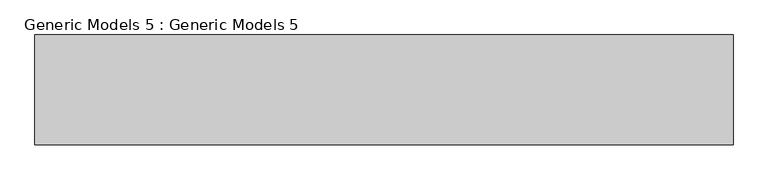
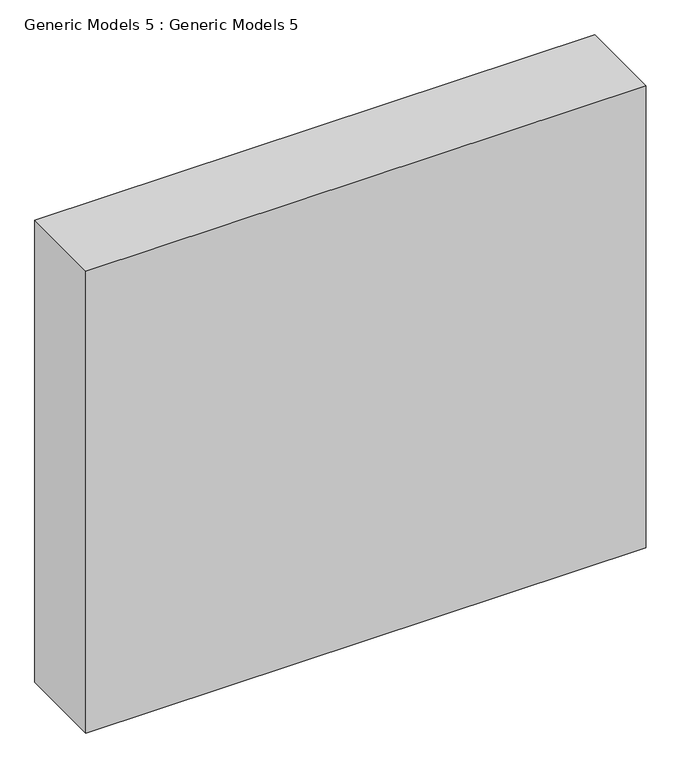
"""IFC4 building model written with IfcOpenShell, lengths in millimetres: proxy geometry, Generic Models 5 : Generic Models 5."""

from ifc_helpers import new_model, si_unit, frame, origin, place, context, project, spatial, polyline, outline, extrude, source, transform, mapped, element, save


def generic_models_5_generic_models_5_710787d1(model_context):
    return source(origin(), model_context, "Body", "SweptSolid", [
        extrude(outline(polyline([(-5051.4108866, -2503.4600272), (-3117.2664982, -2503.4600272), (-3117.2664982, -2808.2600272), (-5051.4108866, -2808.2600272), (-5051.4108866, -2503.4600272)])), frame((0.0, 0.0, 1362.3923044), z_axis=(0.0, 0.0, 1.0), x_axis=(1.0, 0.0, 0.0)), (0.0, 0.0, 1.0), 1685.6076956),
    ])


if __name__ == "__main__":
    model = new_model("IFC4")
    model_context = context("Model", 3, world=origin())
    ifc_project = project(units=[si_unit("LENGTHUNIT", "METRE", prefix="MILLI")], contexts=[model_context])
    site = spatial("IfcSite", under=ifc_project)
    building = spatial("IfcBuilding", under=site)
    placement = place(None, origin())
    generic_models_5_generic_models_5_shape = generic_models_5_generic_models_5_710787d1(model_context)
    element("IfcBuildingElementProxy", 1, Name="Generic Models 5 : Generic Models 5", ObjectType="Generic Models 5 : Generic Models 5", at=placement, inside=building, context=model_context, shape_type="MappedRepresentation", body=[
        mapped(generic_models_5_generic_models_5_shape, transform((0.0, 0.0, 0.0), x_axis=(1.0, 0.0, 0.0), y_axis=(0.0, 1.0, 0.0), z_axis=(0.0, 0.0, 1.0))),
    ])
    save(model, "model.ifc")
